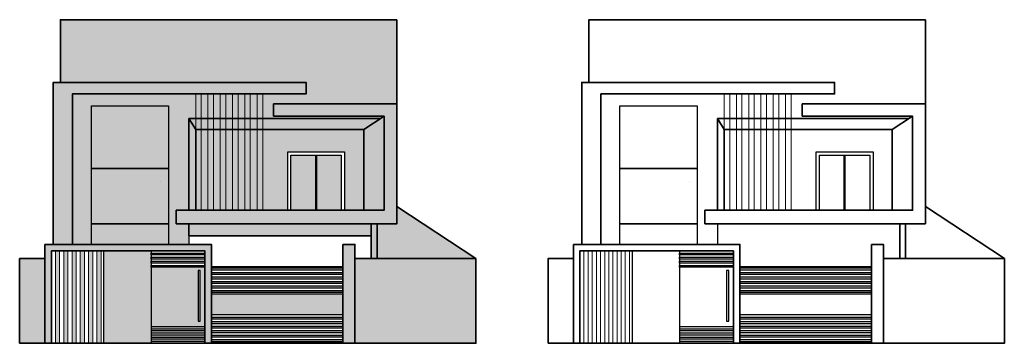
# Model space of a CAD drawing. Units: feet. Extents: x 3882 to 5038, y 866 to 1245.
import ezdxf

# ---------------------------------------------------------------- set-up
doc = ezdxf.new("R2010")
doc.units = ezdxf.units.FT
for name, color, linetype, lineweight in [('A-DOOR', 4, 'Continuous', 25), ('A-ELEV', 7, 'Continuous', 35), ('A-ELEV-FINS', 8, 'Continuous', 18), ('A-ELEV-PATT', 252, 'Continuous', 13), ('A-GLAZ', 4, 'Continuous', 25)]:
    doc.layers.add(name, color=color, linetype=linetype, lineweight=lineweight)

msp = doc.modelspace()

# ---------------------------------------------------------------- hatches: boundary and pattern name
at = {"layer": 'A-ELEV-PATT'}
h = msp.add_hatch(color=256, dxfattribs=at)
h.dxf.hatch_style = 1
h.paths.add_polyline_path([(4324.8, 1245.2), (3929.9, 1245.2), (3929.9, 1171.7), (4218.3, 1171.7), (4218.3, 1158.2), (4167.3, 1158.2), (4167.3, 1129.4), (4305.7, 1129.4), (4309.8, 1132.1), (4180.1, 1132.1), (4180.1, 1146.5), (4324.8, 1146.5)])
h.paths.add_polyline_path([(4080.8, 1129.4), (4088.7, 1129.4), (4088.7, 1158.2), (3944.1, 1158.2), (3944.1, 997.5), (3944.1, 981.8), (3966.4, 981.8), (3966.4, 1144.3), (4056.9, 1144.3), (4056.9, 981.8), (4080.8, 981.8), (4080.8, 1006), (4065.9, 1006), (4065.9, 1021.8), (4080.8, 1021.8)])
h.paths.add_polyline_path([(4095.2, 1158.2), (4088.7, 1158.2), (4088.7, 1129.4), (4095.2, 1129.4)], flags=17)
h.paths.add_polyline_path([(4103.1, 1158.2), (4095.2, 1158.2), (4095.2, 1129.4), (4103.1, 1129.4)], flags=17)
h.paths.add_polyline_path([(4109.6, 1158.2), (4103.1, 1158.2), (4103.1, 1129.4), (4109.6, 1129.4)], flags=17)
h.paths.add_polyline_path([(4117.5, 1158.2), (4109.6, 1158.2), (4109.6, 1129.4), (4117.5, 1129.4)], flags=17)
h.paths.add_polyline_path([(4124, 1158.2), (4117.5, 1158.2), (4117.5, 1129.4), (4124, 1129.4)], flags=17)
h.paths.add_polyline_path([(4131.9, 1158.2), (4124, 1158.2), (4124, 1129.4), (4131.9, 1129.4)], flags=17)
h.paths.add_polyline_path([(4138.4, 1158.2), (4131.9, 1158.2), (4131.9, 1129.4), (4138.4, 1129.4)], flags=17)
h.paths.add_polyline_path([(4146.3, 1158.2), (4138.4, 1158.2), (4138.4, 1129.4), (4146.3, 1129.4)], flags=17)
h.paths.add_polyline_path([(4152.8, 1158.2), (4146.3, 1158.2), (4146.3, 1129.4), (4152.8, 1129.4)], flags=17)
h.paths.add_polyline_path([(4160.8, 1158.2), (4152.8, 1158.2), (4152.8, 1129.4), (4160.8, 1129.4)], flags=17)
h.paths.add_polyline_path([(4167.3, 1158.2), (4160.8, 1158.2), (4160.8, 1129.4), (4167.3, 1129.4)], flags=17)
h.paths.add_polyline_path([(4095.2, 1129.4), (4088.7, 1129.4), (4088.7, 1116.4), (4095.2, 1116.4)])
h.paths.add_polyline_path([(4095.2, 1116.4), (4088.7, 1116.4), (4088.7, 1021.8), (4095.2, 1021.8)])
h.paths.add_polyline_path([(4109.6, 1129.4), (4103.1, 1129.4), (4103.1, 1116.4), (4109.6, 1116.4)])
h.paths.add_polyline_path([(4109.6, 1116.4), (4103.1, 1116.4), (4103.1, 1021.8), (4109.6, 1021.8)])
h.paths.add_polyline_path([(4124, 1129.4), (4117.5, 1129.4), (4117.5, 1116.4), (4124, 1116.4)])
h.paths.add_polyline_path([(4124, 1116.4), (4117.5, 1116.4), (4117.5, 1021.8), (4124, 1021.8)])
h.paths.add_polyline_path([(4138.4, 1129.4), (4131.9, 1129.4), (4131.9, 1116.4), (4138.4, 1116.4)])
h.paths.add_polyline_path([(4138.4, 1116.4), (4131.9, 1116.4), (4131.9, 1021.8), (4138.4, 1021.8)])
h.paths.add_polyline_path([(4152.8, 1129.4), (4146.3, 1129.4), (4146.3, 1116.4), (4152.8, 1116.4)])
h.paths.add_polyline_path([(4152.8, 1116.4), (4146.3, 1116.4), (4146.3, 1021.8), (4152.8, 1021.8)])
h.paths.add_polyline_path([(4167.3, 1129.4), (4160.8, 1129.4), (4160.8, 1116.4), (4167.3, 1116.4)])
h.paths.add_polyline_path([(4167.3, 1116.4), (4160.8, 1116.4), (4160.8, 1021.8), (4167.3, 1021.8)])
h.paths.add_polyline_path([(4301.6, 1006), (4294.7, 1006), (4294.7, 965.1), (4301.6, 965.1)])
h.paths.add_polyline_path([(3929, 974.2), (3924.1, 974.2), (3924.1, 865.8), (3929, 865.8)])
h.paths.add_polyline_path([(3938.7, 974.2), (3933.8, 974.2), (3933.8, 865.8), (3938.7, 865.8)])
h.paths.add_polyline_path([(3948.5, 974.2), (3943.6, 974.2), (3943.6, 865.8), (3948.5, 865.8)])
h.paths.add_polyline_path([(3958.2, 974.2), (3953.3, 974.2), (3953.3, 865.8), (3958.2, 865.8)])
h.paths.add_polyline_path([(3967.9, 974.2), (3963, 974.2), (3963, 865.8), (3967.9, 865.8)])
h.paths.add_polyline_path([(3977.6, 974.2), (3972.7, 974.2), (3972.7, 865.8), (3977.6, 865.8)])
h = msp.add_hatch(color=256, dxfattribs=at)
h.dxf.hatch_style = 1
h.paths.add_polyline_path([(3944.1, 1158.2), (4218.3, 1158.2), (4218.3, 1171.7), (3921.6, 1171.7), (3921.6, 997.5), (3921.6, 981.8), (3944.1, 981.8), (3944.1, 997.5)])
h.paths.add_polyline_path([(4036.4, 974.2), (3981, 974.2), (3981, 865.8), (4036.4, 865.8)])
h = msp.add_hatch(color=256, dxfattribs=at)
h.dxf.hatch_style = 1
h.paths.add_polyline_path([(4324.8, 1146.5), (4180.1, 1146.5), (4180.1, 1132.1), (4309.8, 1132.1), (4309.8, 1021.8), (4301.6, 1021.8), (4080.8, 1021.8), (4065.9, 1021.8), (4065.9, 1006), (4080.8, 1006), (4294.7, 1006), (4324.8, 1006)])
h.paths.add_polyline_path([(4107.1, 981.8), (3911.7, 981.8), (3911.7, 865.8), (3919.3, 865.8), (3919.3, 974.2), (4099.6, 974.2), (4099.6, 865.8), (4107.1, 865.8), (4107.1, 955.6)])
h.paths.add_polyline_path([(4099.6, 954.9), (4036.4, 954.9), (4036.4, 885.2), (4099.6, 885.2)], flags=17)
h.paths.add_polyline_path([(4091.6, 951.3), (4094.1, 951.3), (4094.1, 891.8), (4091.6, 891.8)], flags=16)
h.paths.add_polyline_path([(4099.6, 971.7), (4036.4, 971.7), (4036.4, 969.4), (4099.6, 969.4)], flags=17)
h.paths.add_polyline_path([(4099.6, 966.8), (4036.4, 966.8), (4036.4, 964.6), (4099.6, 964.6)], flags=17)
h.paths.add_polyline_path([(4099.6, 962), (4036.4, 962), (4036.4, 959.7), (4099.6, 959.7)], flags=17)
h.paths.add_polyline_path([(4099.6, 957.2), (4036.4, 957.2), (4036.4, 954.9), (4099.6, 954.9)], flags=17)
h.paths.add_polyline_path([(4275.5, 965.1), (4275.5, 981.8), (4261.5, 981.8), (4261.5, 865.8), (4275.5, 865.8)])
h = msp.add_hatch(color=256, dxfattribs=at)
h.dxf.hatch_style = 1
h.paths.add_polyline_path([(4056.9, 1144.3), (3966.4, 1144.3), (3966.4, 1070.9), (4056.9, 1070.9)])
h.paths.add_polyline_path([(4056.9, 1070.7), (3966.4, 1070.7), (3966.4, 1006), (4056.9, 1006)])
h.paths.add_polyline_path([(4056.9, 1005.8), (3966.4, 1005.8), (3966.4, 981.8), (4056.9, 981.8)])
h.paths.add_polyline_path([(4259.6, 1086.5), (4230.3, 1086.5), (4230.3, 1021.8), (4259.6, 1021.8)])
h.paths.add_polyline_path([(4229.7, 1086.5), (4200.5, 1086.5), (4200.5, 1021.8), (4229.7, 1021.8)])
h = msp.add_hatch(color=256, dxfattribs=at)
h.dxf.hatch_style = 1
h.paths.add_polyline_path([(3911.7, 965.1), (3882.1, 965.1), (3882.1, 865.8), (3911.7, 865.8)])
h.paths.add_polyline_path([(4417.5, 965.1), (4275.5, 965.1), (4275.5, 865.8), (4417.5, 865.8)])
h.paths.add_polyline_path([(4324.8, 1026.2), (4324.8, 1006), (4301.6, 1006), (4301.6, 965.1), (4417.5, 965.1)])
h.paths.add_polyline_path([(4305.7, 1129.4), (4167.3, 1129.4), (4167.3, 1116.4), (4286, 1116.4)])
h.paths.add_polyline_path([(4309.8, 1132.1), (4286, 1116.4), (4286, 1021.8), (4301.6, 1021.8), (4309.8, 1021.8)])
h.paths.add_polyline_path([(4088.7, 1116.4), (4080.8, 1129.4), (4080.8, 1021.8), (4088.7, 1021.8)])
h.paths.add_polyline_path([(4088.7, 1129.4), (4080.8, 1129.4), (4088.7, 1116.4)], flags=17)
h.paths.add_polyline_path([(4103.1, 1129.4), (4095.2, 1129.4), (4095.2, 1116.4), (4103.1, 1116.4)])
h.paths.add_polyline_path([(4117.5, 1129.4), (4109.6, 1129.4), (4109.6, 1116.4), (4117.5, 1116.4)])
h.paths.add_polyline_path([(4131.9, 1129.4), (4124, 1129.4), (4124, 1116.4), (4131.9, 1116.4)])
h.paths.add_polyline_path([(4146.3, 1129.4), (4138.4, 1129.4), (4138.4, 1116.4), (4146.3, 1116.4)])
h.paths.add_polyline_path([(4160.8, 1129.4), (4152.8, 1129.4), (4152.8, 1116.4), (4160.8, 1116.4)])
h = msp.add_hatch(color=256, dxfattribs=at)
h.dxf.hatch_style = 1
h.paths.add_polyline_path([(4196.7, 1090.2), (4263.3, 1090.2), (4263.3, 1021.8), (4286, 1021.8), (4286, 1116.4), (4167.3, 1116.4), (4167.3, 1021.8), (4196.7, 1021.8)])
h.paths.add_polyline_path([(4103.1, 1116.4), (4095.2, 1116.4), (4095.2, 1021.8), (4103.1, 1021.8)])
h.paths.add_polyline_path([(4117.5, 1116.4), (4109.6, 1116.4), (4109.6, 1021.8), (4117.5, 1021.8)])
h.paths.add_polyline_path([(4131.9, 1116.4), (4124, 1116.4), (4124, 1021.8), (4131.9, 1021.8)])
h.paths.add_polyline_path([(4146.3, 1116.4), (4138.4, 1116.4), (4138.4, 1021.8), (4146.3, 1021.8)])
h.paths.add_polyline_path([(4160.8, 1116.4), (4152.8, 1116.4), (4152.8, 1021.8), (4160.8, 1021.8)])
h = msp.add_hatch(color=256, dxfattribs=at)
h.dxf.hatch_style = 1
h.paths.add_polyline_path([(4294.7, 1006), (4080.8, 1006), (4080.8, 991.7), (4294.7, 991.7)])
h = msp.add_hatch(color=256, dxfattribs=at)
h.dxf.hatch_style = 1
h.paths.add_polyline_path([(4099.6, 870.7), (4036.4, 870.7), (4036.4, 868.4), (4099.6, 868.4)])
h.paths.add_polyline_path([(4099.6, 875.5), (4036.4, 875.5), (4036.4, 873.2), (4099.6, 873.2)])
h.paths.add_polyline_path([(4099.6, 880.3), (4036.4, 880.3), (4036.4, 878.1), (4099.6, 878.1)])
h.paths.add_polyline_path([(4099.6, 885.2), (4036.4, 885.2), (4036.4, 882.9), (4099.6, 882.9)])
h.paths.add_polyline_path([(4261.5, 923.8), (4107.1, 923.8), (4107.1, 899.2), (4261.5, 899.2)])
h.paths.add_polyline_path([(4261.5, 896.5), (4107.1, 896.5), (4107.1, 894), (4261.5, 894)])
h.paths.add_polyline_path([(4261.5, 891.2), (4107.1, 891.2), (4107.1, 888.7), (4261.5, 888.7)])
h.paths.add_polyline_path([(4261.5, 885.9), (4107.1, 885.9), (4107.1, 883.4), (4261.5, 883.4)])
h.paths.add_polyline_path([(4261.5, 880.7), (4107.1, 880.7), (4107.1, 878.2), (4261.5, 878.2)])
h.paths.add_polyline_path([(4261.5, 875.4), (4107.1, 875.4), (4107.1, 872.9), (4261.5, 872.9)])
h.paths.add_polyline_path([(4261.5, 870.1), (4107.1, 870.1), (4107.1, 867.6), (4261.5, 867.6)])
h.paths.add_polyline_path([(4261.5, 927.8), (4107.1, 927.8), (4107.1, 925.3), (4261.5, 925.3)])
h.paths.add_polyline_path([(4261.5, 933.1), (4107.1, 933.1), (4107.1, 930.6), (4261.5, 930.6)])
h.paths.add_polyline_path([(4261.5, 938.4), (4107.1, 938.4), (4107.1, 935.9), (4261.5, 935.9)])
h.paths.add_polyline_path([(4261.5, 943.6), (4107.1, 943.6), (4107.1, 941.1), (4261.5, 941.1)])
h.paths.add_polyline_path([(4261.5, 954.2), (4107.1, 954.2), (4107.1, 951.7), (4261.5, 951.7)])
h.paths.add_polyline_path([(4261.5, 948.9), (4107.1, 948.9), (4107.1, 946.4), (4261.5, 946.4)])

# ---------------------------------------------------------------- linework, layer by layer
at = {"layer": 'A-DOOR'}
for points in [[(4196.7, 1090.2), (4263.3, 1090.2), (4263.3, 1021.8), (4196.7, 1021.8)], [(4196.7, 1090.2), (4263.3, 1090.2), (4263.3, 1021.8), (4196.7, 1021.8)], [(4229.7, 1086.5), (4230.3, 1086.5), (4230.3, 1021.8), (4229.7, 1021.8)], [(4229.7, 1086.5), (4230.3, 1086.5), (4230.3, 1021.8), (4229.7, 1021.8)], [(4816.9, 1090.2), (4883.6, 1090.2), (4883.6, 1021.8), (4816.9, 1021.8)], [(4849.9, 1086.5), (4850.5, 1086.5), (4850.5, 1021.8), (4849.9, 1021.8)], [(3981, 974.2), (4036.4, 974.2), (4036.4, 865.8), (3981, 865.8)], [(3981, 974.2), (4036.4, 974.2), (4036.4, 865.8), (3981, 865.8)], [(4036.4, 971.7), (4099.6, 971.7), (4099.6, 969.4), (4036.4, 969.4)], [(4036.4, 971.7), (4099.6, 971.7), (4099.6, 969.4), (4036.4, 969.4)], [(4601.2, 974.2), (4656.6, 974.2), (4656.6, 865.8), (4601.2, 865.8)], [(4656.6, 971.7), (4719.8, 971.7), (4719.8, 969.4), (4656.6, 969.4)], [(4036.4, 966.8), (4099.6, 966.8), (4099.6, 964.6), (4036.4, 964.6)], [(4036.4, 966.8), (4099.6, 966.8), (4099.6, 964.6), (4036.4, 964.6)], [(4036.4, 962), (4099.6, 962), (4099.6, 959.7), (4036.4, 959.7)], [(4036.4, 962), (4099.6, 962), (4099.6, 959.7), (4036.4, 959.7)], [(4656.6, 966.8), (4719.8, 966.8), (4719.8, 964.6), (4656.6, 964.6)], [(4656.6, 962), (4719.8, 962), (4719.8, 959.7), (4656.6, 959.7)], [(4036.4, 957.2), (4099.6, 957.2), (4099.6, 954.9), (4036.4, 954.9)], [(4036.4, 957.2), (4099.6, 957.2), (4099.6, 954.9), (4036.4, 954.9)], [(4094.1, 951.3), (4091.6, 951.3), (4091.6, 891.8), (4094.1, 891.8)], [(4094.1, 951.3), (4091.6, 951.3), (4091.6, 891.8), (4094.1, 891.8)], [(4107.1, 865.8), (4261.5, 865.8), (4261.5, 955.6), (4107.1, 955.6)], [(4107.1, 865.8), (4261.5, 865.8), (4261.5, 955.6), (4107.1, 955.6)], [(4107.1, 954.2), (4261.5, 954.2), (4261.5, 951.7), (4107.1, 951.7)], [(4107.1, 954.2), (4261.5, 954.2), (4261.5, 951.7), (4107.1, 951.7)], [(4107.1, 948.9), (4261.5, 948.9), (4261.5, 946.4), (4107.1, 946.4)], [(4107.1, 948.9), (4261.5, 948.9), (4261.5, 946.4), (4107.1, 946.4)], [(4656.6, 957.2), (4719.8, 957.2), (4719.8, 954.9), (4656.6, 954.9)], [(4714.3, 951.3), (4711.8, 951.3), (4711.8, 891.8), (4714.3, 891.8)], [(4727.3, 865.8), (4881.7, 865.8), (4881.7, 955.6), (4727.3, 955.6)], [(4727.3, 954.2), (4881.7, 954.2), (4881.7, 951.7), (4727.3, 951.7)], [(4727.3, 948.9), (4881.7, 948.9), (4881.7, 946.4), (4727.3, 946.4)], [(4107.1, 943.6), (4261.5, 943.6), (4261.5, 941.1), (4107.1, 941.1)], [(4107.1, 943.6), (4261.5, 943.6), (4261.5, 941.1), (4107.1, 941.1)], [(4107.1, 938.4), (4261.5, 938.4), (4261.5, 935.9), (4107.1, 935.9)], [(4107.1, 938.4), (4261.5, 938.4), (4261.5, 935.9), (4107.1, 935.9)], [(4727.3, 943.6), (4881.7, 943.6), (4881.7, 941.1), (4727.3, 941.1)], [(4727.3, 938.4), (4881.7, 938.4), (4881.7, 935.9), (4727.3, 935.9)], [(4107.1, 933.1), (4261.5, 933.1), (4261.5, 930.6), (4107.1, 930.6)], [(4107.1, 933.1), (4261.5, 933.1), (4261.5, 930.6), (4107.1, 930.6)], [(4107.1, 927.8), (4261.5, 927.8), (4261.5, 925.3), (4107.1, 925.3)], [(4107.1, 927.8), (4261.5, 927.8), (4261.5, 925.3), (4107.1, 925.3)], [(4727.3, 933.1), (4881.7, 933.1), (4881.7, 930.6), (4727.3, 930.6)], [(4727.3, 927.8), (4881.7, 927.8), (4881.7, 925.3), (4727.3, 925.3)], [(4107.1, 923.8), (4261.5, 923.8), (4261.5, 899.2), (4107.1, 899.2)], [(4107.1, 923.8), (4261.5, 923.8), (4261.5, 899.2), (4107.1, 899.2)], [(4727.3, 923.8), (4881.7, 923.8), (4881.7, 899.2), (4727.3, 899.2)], [(4107.1, 896.5), (4261.5, 896.5), (4261.5, 894), (4107.1, 894)], [(4107.1, 896.5), (4261.5, 896.5), (4261.5, 894), (4107.1, 894)], [(4107.1, 891.2), (4261.5, 891.2), (4261.5, 888.7), (4107.1, 888.7)], [(4107.1, 891.2), (4261.5, 891.2), (4261.5, 888.7), (4107.1, 888.7)], [(4727.3, 896.5), (4881.7, 896.5), (4881.7, 894), (4727.3, 894)], [(4727.3, 891.2), (4881.7, 891.2), (4881.7, 888.7), (4727.3, 888.7)], [(4036.4, 882.9), (4099.6, 882.9), (4099.6, 885.2), (4036.4, 885.2)], [(4036.4, 882.9), (4099.6, 882.9), (4099.6, 885.2), (4036.4, 885.2)], [(4036.4, 878.1), (4099.6, 878.1), (4099.6, 880.3), (4036.4, 880.3)], [(4036.4, 878.1), (4099.6, 878.1), (4099.6, 880.3), (4036.4, 880.3)], [(4107.1, 885.9), (4261.5, 885.9), (4261.5, 883.4), (4107.1, 883.4)], [(4107.1, 885.9), (4261.5, 885.9), (4261.5, 883.4), (4107.1, 883.4)], [(4107.1, 880.7), (4261.5, 880.7), (4261.5, 878.2), (4107.1, 878.2)], [(4107.1, 880.7), (4261.5, 880.7), (4261.5, 878.2), (4107.1, 878.2)], [(4656.6, 882.9), (4719.8, 882.9), (4719.8, 885.2), (4656.6, 885.2)], [(4656.6, 878.1), (4719.8, 878.1), (4719.8, 880.3), (4656.6, 880.3)], [(4727.3, 885.9), (4881.7, 885.9), (4881.7, 883.4), (4727.3, 883.4)], [(4727.3, 880.7), (4881.7, 880.7), (4881.7, 878.2), (4727.3, 878.2)], [(4036.4, 873.2), (4099.6, 873.2), (4099.6, 875.5), (4036.4, 875.5)], [(4036.4, 873.2), (4099.6, 873.2), (4099.6, 875.5), (4036.4, 875.5)], [(4036.4, 868.4), (4099.6, 868.4), (4099.6, 870.7), (4036.4, 870.7)], [(4036.4, 868.4), (4099.6, 868.4), (4099.6, 870.7), (4036.4, 870.7)], [(4107.1, 875.4), (4261.5, 875.4), (4261.5, 872.9), (4107.1, 872.9)], [(4107.1, 875.4), (4261.5, 875.4), (4261.5, 872.9), (4107.1, 872.9)], [(4107.1, 870.1), (4261.5, 870.1), (4261.5, 867.6), (4107.1, 867.6)], [(4107.1, 870.1), (4261.5, 870.1), (4261.5, 867.6), (4107.1, 867.6)], [(4656.6, 873.2), (4719.8, 873.2), (4719.8, 875.5), (4656.6, 875.5)], [(4656.6, 868.4), (4719.8, 868.4), (4719.8, 870.7), (4656.6, 870.7)], [(4727.3, 875.4), (4881.7, 875.4), (4881.7, 872.9), (4727.3, 872.9)], [(4727.3, 870.1), (4881.7, 870.1), (4881.7, 867.6), (4727.3, 867.6)]]:
    msp.add_lwpolyline(points, close=True, dxfattribs=at)
for points in [[(4200.5, 1021.8), (4200.5, 1086.5), (4259.6, 1086.5), (4259.6, 1021.8)], [(4200.5, 1021.8), (4200.5, 1086.5), (4259.6, 1086.5), (4259.6, 1021.8)], [(4820.7, 1021.8), (4820.7, 1086.5), (4879.8, 1086.5), (4879.8, 1021.8)]]:
    msp.add_lwpolyline(points, dxfattribs=at)
at = {"layer": 'A-ELEV'}
for p, q in [((4324.8, 1245.2), (4324.8, 1146.5)), ((4324.8, 1245.2), (4324.8, 1146.5)), ((4945, 1245.2), (4945, 1146.5)), ((4180.1, 1146.5), (4180.1, 1132.1)), ((4180.1, 1146.5), (4180.1, 1132.1)), ((4800.3, 1146.5), (4800.3, 1132.1)), ((4305.7, 1129.4), (4080.8, 1129.4)), ((4080.8, 1129.4), (4088.7, 1116.4)), ((4305.7, 1129.4), (4080.8, 1129.4)), ((4080.8, 1129.4), (4088.7, 1116.4)), ((4286, 1116.4), (4309.8, 1132.1)), ((4286, 1116.4), (4309.8, 1132.1)), ((4925.9, 1129.4), (4701, 1129.4)), ((4701, 1129.4), (4708.9, 1116.4)), ((4906.2, 1116.4), (4930, 1132.1)), ((4065.9, 1021.8), (4065.9, 1006)), ((4065.9, 1021.8), (4065.9, 1006)), ((4417.5, 965.1), (4324.8, 1026.2)), ((4417.5, 965.1), (4324.8, 1026.2)), ((4686.1, 1021.8), (4686.1, 1006)), ((5037.7, 965.1), (4945, 1026.2)), ((3882.1, 865.8), (4417.5, 865.8)), ((3882.1, 865.8), (4417.5, 865.8)), ((4502.3, 865.8), (5037.7, 865.8))]:
    msp.add_line(p, q, dxfattribs=at)
for points in [[(4324.8, 1245.2), (3929.9, 1245.2), (3929.9, 1171.7)], [(4324.8, 1245.2), (3929.9, 1245.2), (3929.9, 1171.7)], [(4945, 1245.2), (4550.1, 1245.2), (4550.1, 1171.7)], [(3921.6, 1171.7), (3929.9, 1171.7)], [(3921.6, 1171.7), (3929.9, 1171.7)], [(4541.8, 1171.7), (4550.1, 1171.7)], [(4180.1, 1146.5), (4324.8, 1146.5), (4324.8, 1006), (4294.7, 1006)], [(4180.1, 1146.5), (4324.8, 1146.5), (4324.8, 1006), (4294.7, 1006)], [(4800.3, 1146.5), (4945, 1146.5), (4945, 1006), (4914.9, 1006)], [(4080.8, 1129.4), (4080.8, 1021.8)], [(4080.8, 1129.4), (4080.8, 1021.8)], [(4301.6, 1021.8), (4309.8, 1021.8), (4309.8, 1132.1), (4180.1, 1132.1)], [(4301.6, 1021.8), (4309.8, 1021.8), (4309.8, 1132.1), (4180.1, 1132.1)], [(4701, 1129.4), (4701, 1021.8)], [(4921.8, 1021.8), (4930, 1021.8), (4930, 1132.1), (4800.3, 1132.1)], [(4047.9, 1055), (4047.9, 1055.2)], [(4047.9, 1055), (4047.9, 1055.2)], [(4668.1, 1055), (4668.1, 1055.2)], [(4065.9, 1021.8), (4080.8, 1021.8)], [(4065.9, 1021.8), (4080.8, 1021.8)], [(4301.6, 1021.8), (4080.8, 1021.8)], [(4301.6, 1021.8), (4080.8, 1021.8)], [(4686.1, 1021.8), (4701, 1021.8)], [(4921.8, 1021.8), (4701, 1021.8)], [(4080.8, 1006), (4065.9, 1006)], [(4080.8, 1006), (4065.9, 1006)], [(4080.8, 1006), (4294.7, 1006)], [(4080.8, 1006), (4294.7, 1006)], [(4294.7, 1006), (4294.7, 965.1), (4301.6, 965.1)], [(4294.7, 1006), (4294.7, 965.1), (4301.6, 965.1)], [(4301.6, 965.1), (4301.6, 1006)], [(4301.6, 965.1), (4301.6, 1006)], [(4701, 1006), (4686.1, 1006)], [(4701, 1006), (4914.9, 1006)], [(4914.9, 1006), (4914.9, 965.1), (4921.8, 965.1)], [(4921.8, 965.1), (4921.8, 1006)], [(4099.6, 865.8), (4099.6, 974.2), (3919.3, 974.2), (3919.3, 865.8)], [(4099.6, 865.8), (4099.6, 974.2), (3919.3, 974.2), (3919.3, 865.8)], [(4719.8, 865.8), (4719.8, 974.2), (4539.5, 974.2), (4539.5, 865.8)]]:
    msp.add_lwpolyline(points, dxfattribs=at)
for points in [[(3921.6, 997.5), (3921.6, 981.8), (3944.1, 981.8), (3944.1, 997.5), (3944.1, 1158.2), (4218.3, 1158.2), (4218.3, 1171.7), (3921.6, 1171.7)], [(3921.6, 997.5), (3921.6, 981.8), (3944.1, 981.8), (3944.1, 997.5), (3944.1, 1158.2), (4218.3, 1158.2), (4218.3, 1171.7), (3921.6, 1171.7)], [(4541.8, 997.5), (4541.8, 981.8), (4564.3, 981.8), (4564.3, 997.5), (4564.3, 1158.2), (4838.5, 1158.2), (4838.5, 1171.7), (4541.8, 1171.7)], [(4286, 1021.8), (4088.7, 1021.8), (4088.7, 1116.4), (4286, 1116.4)], [(4286, 1021.8), (4088.7, 1021.8), (4088.7, 1116.4), (4286, 1116.4)], [(4906.2, 1021.8), (4708.9, 1021.8), (4708.9, 1116.4), (4906.2, 1116.4)], [(3966.4, 1070.9), (4056.9, 1070.9), (4056.9, 1070.7), (3966.4, 1070.7)], [(3966.4, 1070.9), (4056.9, 1070.9), (4056.9, 1070.7), (3966.4, 1070.7)], [(4586.6, 1070.9), (4677.1, 1070.9), (4677.1, 1070.7), (4586.6, 1070.7)], [(4080.8, 1006), (4294.7, 1006), (4294.7, 991.7), (4080.8, 991.7)], [(3911.7, 981.8), (4107.1, 981.8), (4107.1, 865.8), (3911.7, 865.8)], [(3911.7, 981.8), (4107.1, 981.8), (4107.1, 865.8), (3911.7, 865.8)], [(4261.5, 981.8), (4275.5, 981.8), (4275.5, 865.8), (4261.5, 865.8)], [(4261.5, 981.8), (4275.5, 981.8), (4275.5, 865.8), (4261.5, 865.8)], [(4531.9, 981.8), (4727.3, 981.8), (4727.3, 865.8), (4531.9, 865.8)], [(4881.7, 981.8), (4895.7, 981.8), (4895.7, 865.8), (4881.7, 865.8)], [(3882.1, 865.8), (3911.7, 865.8), (3911.7, 965.1), (3882.1, 965.1)], [(3882.1, 865.8), (3911.7, 865.8), (3911.7, 965.1), (3882.1, 965.1)], [(4417.5, 965.1), (4275.5, 965.1), (4275.5, 865.8), (4417.5, 865.8)], [(4417.5, 965.1), (4275.5, 965.1), (4275.5, 865.8), (4417.5, 865.8)], [(4502.3, 865.8), (4531.9, 865.8), (4531.9, 965.1), (4502.3, 965.1)], [(5037.7, 965.1), (4895.7, 965.1), (4895.7, 865.8), (5037.7, 865.8)]]:
    msp.add_lwpolyline(points, close=True, dxfattribs=at)
at = {"layer": 'A-ELEV-FINS'}
for points in [[(4088.7, 1158.2), (4095.2, 1158.2), (4095.2, 1021.8), (4088.7, 1021.8)], [(4088.7, 1158.2), (4095.2, 1158.2), (4095.2, 1021.8), (4088.7, 1021.8)], [(4103.1, 1158.2), (4109.6, 1158.2), (4109.6, 1021.8), (4103.1, 1021.8)], [(4103.1, 1158.2), (4109.6, 1158.2), (4109.6, 1021.8), (4103.1, 1021.8)], [(4117.5, 1158.2), (4124, 1158.2), (4124, 1021.8), (4117.5, 1021.8)], [(4117.5, 1158.2), (4124, 1158.2), (4124, 1021.8), (4117.5, 1021.8)], [(4131.9, 1158.2), (4138.4, 1158.2), (4138.4, 1021.8), (4131.9, 1021.8)], [(4131.9, 1158.2), (4138.4, 1158.2), (4138.4, 1021.8), (4131.9, 1021.8)], [(4146.3, 1158.2), (4152.8, 1158.2), (4152.8, 1021.8), (4146.3, 1021.8)], [(4146.3, 1158.2), (4152.8, 1158.2), (4152.8, 1021.8), (4146.3, 1021.8)], [(4160.8, 1158.2), (4167.3, 1158.2), (4167.3, 1021.8), (4160.8, 1021.8)], [(4160.8, 1158.2), (4167.3, 1158.2), (4167.3, 1021.8), (4160.8, 1021.8)], [(4708.9, 1158.2), (4715.4, 1158.2), (4715.4, 1021.8), (4708.9, 1021.8)], [(4723.3, 1158.2), (4729.8, 1158.2), (4729.8, 1021.8), (4723.3, 1021.8)], [(4737.7, 1158.2), (4744.2, 1158.2), (4744.2, 1021.8), (4737.7, 1021.8)], [(4752.1, 1158.2), (4758.6, 1158.2), (4758.6, 1021.8), (4752.1, 1021.8)], [(4766.5, 1158.2), (4773, 1158.2), (4773, 1021.8), (4766.5, 1021.8)], [(4781, 1158.2), (4787.5, 1158.2), (4787.5, 1021.8), (4781, 1021.8)], [(3924.1, 974.2), (3929, 974.2), (3929, 865.8), (3924.1, 865.8)], [(3924.1, 974.2), (3929, 974.2), (3929, 865.8), (3924.1, 865.8)], [(3933.8, 974.2), (3938.7, 974.2), (3938.7, 865.8), (3933.8, 865.8)], [(3933.8, 974.2), (3938.7, 974.2), (3938.7, 865.8), (3933.8, 865.8)], [(3943.6, 974.2), (3948.5, 974.2), (3948.5, 865.8), (3943.6, 865.8)], [(3943.6, 974.2), (3948.5, 974.2), (3948.5, 865.8), (3943.6, 865.8)], [(3953.3, 974.2), (3958.2, 974.2), (3958.2, 865.8), (3953.3, 865.8)], [(3953.3, 974.2), (3958.2, 974.2), (3958.2, 865.8), (3953.3, 865.8)], [(3963, 974.2), (3967.9, 974.2), (3967.9, 865.8), (3963, 865.8)], [(3963, 974.2), (3967.9, 974.2), (3967.9, 865.8), (3963, 865.8)], [(3972.7, 974.2), (3977.6, 974.2), (3977.6, 865.8), (3972.7, 865.8)], [(3972.7, 974.2), (3977.6, 974.2), (3977.6, 865.8), (3972.7, 865.8)], [(4544.3, 974.2), (4549.2, 974.2), (4549.2, 865.8), (4544.3, 865.8)], [(4554, 974.2), (4558.9, 974.2), (4558.9, 865.8), (4554, 865.8)], [(4563.8, 974.2), (4568.7, 974.2), (4568.7, 865.8), (4563.8, 865.8)], [(4573.5, 974.2), (4578.4, 974.2), (4578.4, 865.8), (4573.5, 865.8)], [(4583.2, 974.2), (4588.1, 974.2), (4588.1, 865.8), (4583.2, 865.8)], [(4592.9, 974.2), (4597.8, 974.2), (4597.8, 865.8), (4592.9, 865.8)]]:
    msp.add_lwpolyline(points, close=True, dxfattribs=at)
at = {"layer": 'A-GLAZ'}
for points in [[(3966.4, 981.8), (3966.4, 1144.3), (4056.9, 1144.3), (4056.9, 981.8)], [(3966.4, 981.8), (3966.4, 1144.3), (4056.9, 1144.3), (4056.9, 981.8)], [(4586.6, 981.8), (4586.6, 1144.3), (4677.1, 1144.3), (4677.1, 981.8)], [(4080.8, 1006), (4080.8, 981.8)], [(4080.8, 1006), (4080.8, 981.8)], [(4701, 1006), (4701, 981.8)]]:
    msp.add_lwpolyline(points, dxfattribs=at)
for points in [[(3966.4, 1006), (4056.9, 1006), (4056.9, 1005.8), (3966.4, 1005.8)], [(3966.4, 1006), (4056.9, 1006), (4056.9, 1005.8), (3966.4, 1005.8)], [(4586.6, 1006), (4677.1, 1006), (4677.1, 1005.8), (4586.6, 1005.8)]]:
    msp.add_lwpolyline(points, close=True, dxfattribs=at)

doc.saveas('drawing.dxf')
